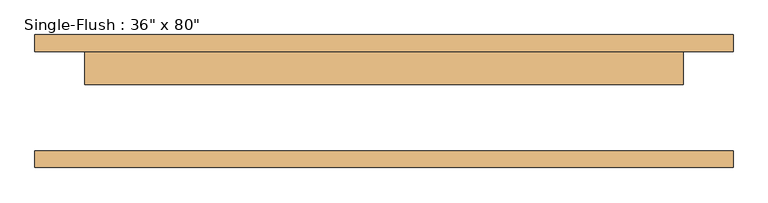
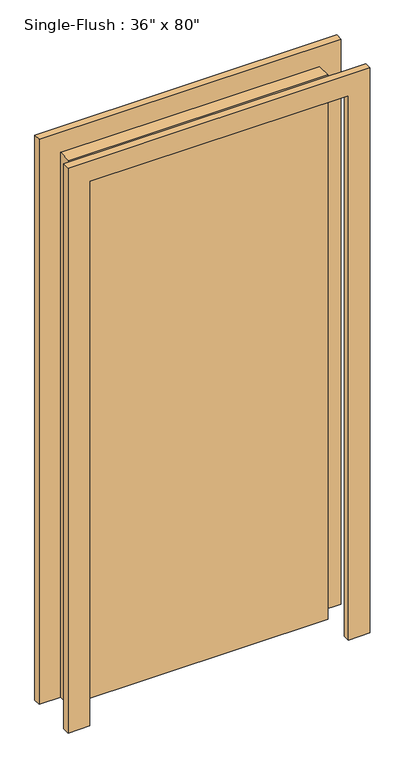
"""IFC4 building model written with IfcOpenShell, lengths in millimetres: door geometry."""

from ifc_helpers import new_model, si_unit, frame, origin, origin_with_axes, place, context, project, spatial, polyline, outline, extrude, source, transform, mapped, element, save


def door_193fcfdc(model_context):
    return source(origin(), model_context, "Body", "SweptSolid", [
        extrude(outline(polyline([(2108.2, -533.4), (0.0, -533.4), (0.0, -457.2), (2032.0, -457.2), (2032.0, 457.2), (0.0, 457.2), (0.0, 533.4), (2108.2, 533.4), (2108.2, -533.4)])), frame((0.0, 76.2, 0.0), z_axis=(0.0, 1.0, 0.0), x_axis=(0.0, 0.0, 1.0)), (0.0, 0.0, 1.0), 25.4),
        extrude(outline(polyline([(2108.2, 533.4), (2108.2, -533.4), (0.0, -533.4), (0.0, -457.2), (2032.0, -457.2), (2032.0, 457.2), (0.0, 457.2), (0.0, 533.4), (2108.2, 533.4)])), frame((0.0, -101.6, 0.0), z_axis=(0.0, 1.0, 0.0), x_axis=(0.0, 0.0, 1.0)), (0.0, 0.0, 1.0), 25.4),
        extrude(outline(polyline([(457.2, 25.4), (-457.2, 25.4), (-457.2, 76.2), (457.2, 76.2), (457.2, 25.4)])), origin_with_axes(), (0.0, 0.0, 1.0), 2032.0),
    ])


if __name__ == "__main__":
    model = new_model("IFC4")
    model_context = context("Model", 3, world=origin())
    ifc_project = project(units=[si_unit("LENGTHUNIT", "METRE", prefix="MILLI")], contexts=[model_context])
    site = spatial("IfcSite", under=ifc_project)
    building = spatial("IfcBuilding", under=site)
    placement = place(None, origin())
    door_shape = door_193fcfdc(model_context)
    element("IfcDoor", 1, ObjectType="Single-Flush : 36\" x 80\"", at=placement, inside=building, context=model_context, shape_type="MappedRepresentation", body=[
        mapped(door_shape, transform((0.0, 0.0, 0.0), x_axis=(1.0, 0.0, 0.0), y_axis=(0.0, 1.0, 0.0), z_axis=(0.0, 0.0, 1.0))),
    ])
    save(model, "model.ifc")

# Revit data of these elements
# Type "Single-Flush : 36\" x 80\""
#   Type Mark = "6"
#   Construction Type Id = "MDOOR"
#   Assembly Code = "C1020"
#   Analytic Construction = "Metal"
#   Thickness = 0' - 2"
#   Heat Transfer Coefficient (U) = 0.651978 BTU/(h·ft²·°F)
#   Height = 6' - 8"
#   Trim Projection Ext = 0' - 1"
#   Trim Projection Int = 0' - 1"
#   Trim Width = 0' - 3"
#   Width = 3' - 0"
#   Define Thermal Properties by = 1
#   Door Material = Door - Panel
#   Frame Material = Door - Frame
#   Visual Light Transmittance = 0
#   Solar Heat Gain Coefficient = 0
#   Function = (empty or 0)
#   Wall Closure = (empty or 0)
# Element 1 (IfcDoor, "Single-Flush : 36\" x 80\"")
#   Materials on its faces: "Door - Frame", "Door - Panel"
# Materials
#   "Door - Panel": class "Wood", colour RGB 210 159 95, transparency 0
#   "Door - Frame": colour RGB 118 70 51, transparency 0
